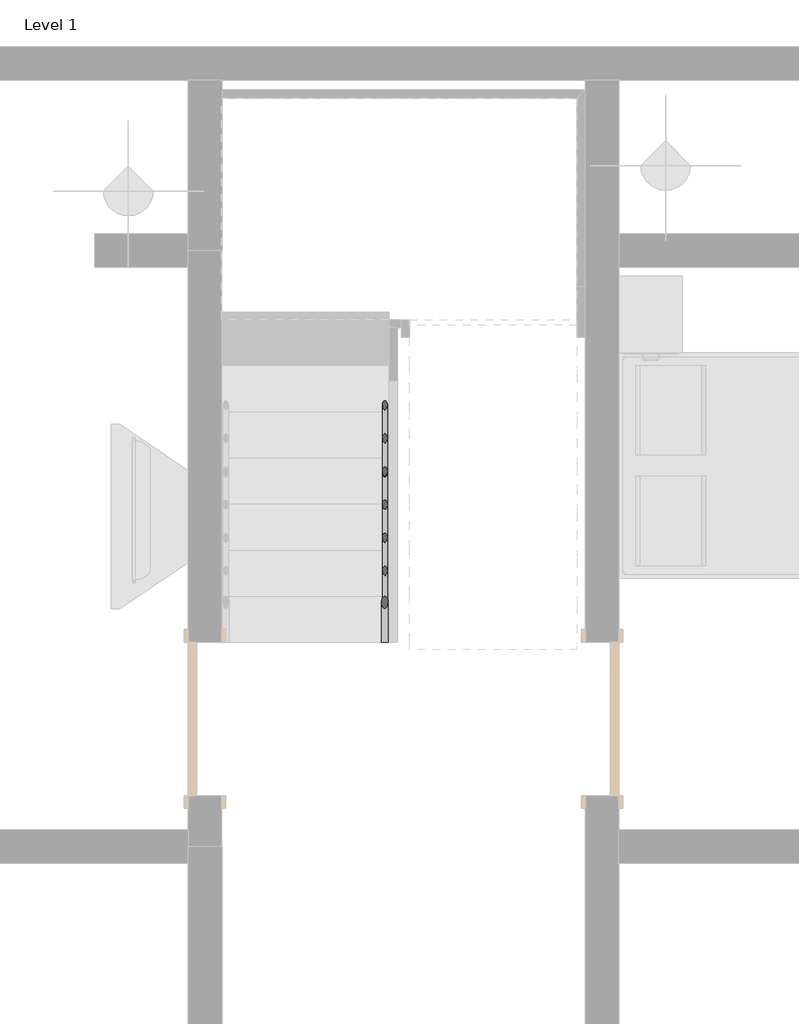
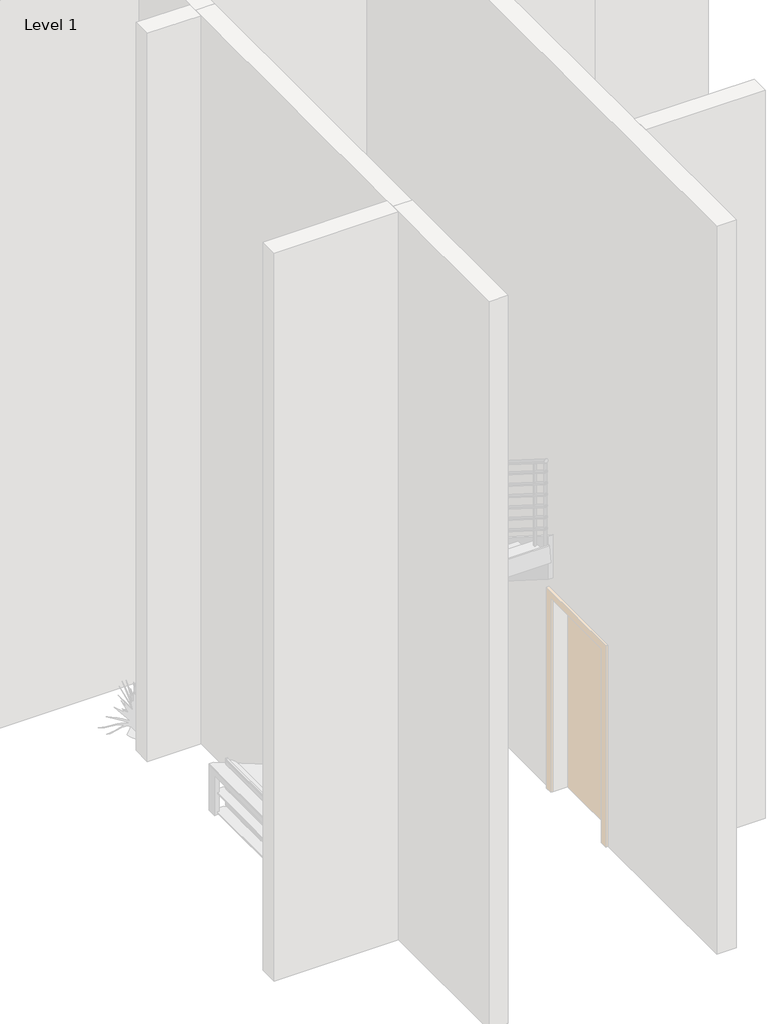
# One storey, part 2 of 4: 1 railing.
"""IFC4 building model written with IfcOpenShell, lengths in millimetres."""

from ifc_helpers import new_model, si_unit, point, frame, frame_2d, origin, place, context, project, spatial, circle_curve, ellipse_curve, trimmed, segment, composite_curve, outline, extrude, element, save
from ifc_brep_helpers import plane_surface, cylinder_surface, advanced_brep

model = new_model("IFC4")

# Units and contexts
model_context = context("Model", 3, world=origin())
ifc_project = project(units=[si_unit("LENGTHUNIT", "METRE", prefix="MILLI")], contexts=[model_context])

# Site, building, storey
site = spatial("IfcSite", under=ifc_project)
building = spatial("IfcBuilding", under=site)
storey = spatial("IfcBuildingStorey", under=building, Name="Level 1", Elevation=0.0)

# Railing
placement = place(None, origin())
element("IfcRailing", 1, ObjectType="900mm Pipe", at=placement, inside=storey, context=model_context, shape_type="SolidModel", body=[
    advanced_brep(
    [(-3568.2939506, 8898.7482221, 1050.2491997), (-3608.2939506, 8898.7482221, 1050.2491997), (-3568.2939506, 10842.9347103, 2279.7742515), (-3608.2939506, 10876.7415595, 2301.1540771)],
    [
        (0, 1, ellipse_curve(frame((-3588.2939506, 8898.7482221, 1050.2491997), z_axis=(0.0, -1.0, 0.0), x_axis=(0.0, 0.0, -1.0)), 23.6638438, 20.0)),
        (1, 0, ellipse_curve(frame((-3588.2939506, 8898.7482221, 1050.2491997), z_axis=(0.0, -1.0, 0.0), x_axis=(0.0, 0.0, -1.0)), 23.6638438, 20.0)),
        (2, 3, ellipse_curve(frame((-3588.2939506, 10859.8381349, 2290.4641643), z_axis=(0.7071067811865479, 0.5976263089853412, 0.37794549184843723), x_axis=(0.7071067811865474, -0.5976263089853417, -0.37794549184843734)), 28.2842712, 20.0)),
        (3, 2, ellipse_curve(frame((-3588.2939506, 10859.8381349, 2290.4641643), z_axis=(0.7071067811865479, 0.5976263089853412, 0.37794549184843723), x_axis=(0.7071067811865474, -0.5976263089853417, -0.37794549184843734)), 28.2842712, 20.0)),
        (0, 2),
        (3, 1),
    ],
    [
        plane_surface(frame((-3588.2939506, 8898.7482221, 1073.9130435), z_axis=(0.0, -1.0, 0.0), x_axis=(0.0, 0.0, 1.0))),
        plane_surface(frame((-3588.2939506, 10849.1482221, 2307.3675889), z_axis=(0.7071067811865479, 0.5976263089853412, 0.37794549184843723), x_axis=(0.7071067811865472, -0.5976263089853417, -0.37794549184843756))),
        cylinder_surface(frame((-3588.2939506, 8909.4381349, 1057.0096189), z_axis=(0.0, -0.8451712313980438, -0.5344956404098301), x_axis=(-1.0, 0.0, 0.0)), 20.0),
    ],
    [
        (0, [[1, 2]]),
        (1, [[3, 4]]),
        (2, [[-1, 5, -4, 6]]),
        (2, [[-2, -6, -3, -5]]),
    ],
),
    advanced_brep(
    [(-3560.7006131, 10829.1482221, 2271.3043478), (-3594.5074624, 10869.1482221, 2271.3043478), (-3414.8939506, 10829.1482221, 2271.3043478), (-3414.8939506, 10869.1482221, 2271.3043478)],
    [
        (0, 1, ellipse_curve(frame((-3577.6040377, 10849.1482221, 2271.3043478), z_axis=(-0.7071067811865479, -0.5976263089853412, -0.37794549184843723), x_axis=(-0.707106781186547, 0.5976263089853417, 0.37794549184843756)), 28.2842712, 20.0)),
        (1, 0, ellipse_curve(frame((-3577.6040377, 10849.1482221, 2271.3043478), z_axis=(-0.7071067811865479, -0.5976263089853412, -0.37794549184843723), x_axis=(-0.707106781186547, 0.5976263089853417, 0.37794549184843756)), 28.2842712, 20.0)),
        (2, 3, ellipse_curve(frame((-3414.8939506, 10849.1482221, 2271.3043478), z_axis=(0.7071067811865476, 0.0, 0.7071067811865476), x_axis=(-0.7071067811865474, 0.0, 0.7071067811865476)), 28.2842712, 20.0)),
        (3, 2, ellipse_curve(frame((-3414.8939506, 10849.1482221, 2271.3043478), z_axis=(0.7071067811865476, 0.0, 0.7071067811865476), x_axis=(-0.7071067811865474, 0.0, 0.7071067811865476)), 28.2842712, 20.0)),
        (0, 2),
        (3, 1),
    ],
    [
        plane_surface(frame((-3588.2939506, 10849.1482221, 2291.3043478), z_axis=(-0.7071067811865479, -0.5976263089853412, -0.37794549184843723), x_axis=(0.7071067811865472, -0.5976263089853417, -0.37794549184843756))),
        plane_surface(frame((-3434.8939506, 10849.1482221, 2291.3043478), z_axis=(0.7071067811865476, 0.0, 0.7071067811865476), x_axis=(0.7071067811865476, 0.0, -0.7071067811865476))),
        cylinder_surface(frame((-3588.2939506, 10849.1482221, 2271.3043478), z_axis=(-1.0, 0.0, 0.0), x_axis=(0.0, 1.0, 0.0)), 20.0),
    ],
    [
        (0, [[1, 2]]),
        (1, [[3, 4]]),
        (2, [[-1, 5, -4, 6]]),
        (2, [[-2, -6, -3, -5]]),
    ],
),
    advanced_brep(
    [(-3414.8939506, 10829.1482221, 2271.3043478), (-3414.8939506, 10869.1482221, 2271.3043478), (-3414.8939506, 10829.1482221, 2414.474684), (-3414.8939506, 10869.1482221, 2436.5059289)],
    [
        (0, 1, ellipse_curve(frame((-3414.8939506, 10849.1482221, 2271.3043478), z_axis=(-0.7071067811865476, 0.0, -0.7071067811865476), x_axis=(0.7071067811865476, 0.0, -0.7071067811865474)), 28.2842712, 20.0)),
        (1, 0, ellipse_curve(frame((-3414.8939506, 10849.1482221, 2271.3043478), z_axis=(-0.7071067811865476, 0.0, -0.7071067811865476), x_axis=(0.7071067811865476, 0.0, -0.7071067811865474)), 28.2842712, 20.0)),
        (2, 3, ellipse_curve(frame((-3414.8939506, 10849.1482221, 2425.4903064), z_axis=(0.0, -0.482443965445817, 0.8759268349610687), x_axis=(0.0, -0.8759268349610687, -0.48244396544581697)), 22.8329573, 20.0)),
        (3, 2, ellipse_curve(frame((-3414.8939506, 10849.1482221, 2425.4903064), z_axis=(0.0, -0.482443965445817, 0.8759268349610687), x_axis=(0.0, -0.8759268349610687, -0.48244396544581697)), 22.8329573, 20.0)),
        (0, 2),
        (3, 1),
    ],
    [
        plane_surface(frame((-3414.8939506, 10849.1482221, 2271.3043478), z_axis=(-0.7071067811865476, 0.0, -0.7071067811865476), x_axis=(0.7071067811865476, 0.0, -0.7071067811865476))),
        plane_surface(frame((-3414.8939506, 10849.1482221, 2425.4903064), z_axis=(0.0, -0.482443965445817, 0.8759268349610687), x_axis=(1.0, 0.0, 0.0))),
        cylinder_surface(frame((-3414.8939506, 10849.1482221, 2271.3043478), z_axis=(0.0, 0.0, -1.0), x_axis=(0.0, 1.0, 0.0)), 20.0),
    ],
    [
        (0, [[1, 2]]),
        (1, [[3, 4]]),
        (2, [[-1, 5, -4, 6]]),
        (2, [[-2, -6, -3, -5]]),
    ],
),
    advanced_brep(
    [(-3434.8939506, 10849.1482221, 2425.4903064), (-3394.8939506, 10849.1482221, 2425.4903064), (-3434.8939506, 8898.7482221, 3658.9448519), (-3394.8939506, 8898.7482221, 3658.9448519)],
    [
        (0, 1, ellipse_curve(frame((-3414.8939506, 10849.1482221, 2425.4903064), z_axis=(0.0, 0.482443965445817, -0.8759268349610687), x_axis=(0.0, 0.8759268349610686, 0.48244396544581697)), 22.8329573, 20.0)),
        (1, 0, ellipse_curve(frame((-3414.8939506, 10849.1482221, 2425.4903064), z_axis=(0.0, 0.482443965445817, -0.8759268349610687), x_axis=(0.0, 0.8759268349610686, 0.48244396544581697)), 22.8329573, 20.0)),
        (2, 3, ellipse_curve(frame((-3414.8939506, 8898.7482221, 3658.9448519), z_axis=(0.0, -1.0, 0.0), x_axis=(0.0, 0.0, -1.0)), 23.6638438, 20.0)),
        (3, 2, ellipse_curve(frame((-3414.8939506, 8898.7482221, 3658.9448519), z_axis=(0.0, -1.0, 0.0), x_axis=(0.0, 0.0, -1.0)), 23.6638438, 20.0)),
        (0, 2),
        (3, 1),
    ],
    [
        plane_surface(frame((-3414.8939506, 10869.1482221, 2436.5059289), z_axis=(0.0, 0.482443965445817, -0.8759268349610687), x_axis=(1.0, 0.0, 0.0))),
        plane_surface(frame((-3414.8939506, 8898.7482221, 3682.6086957), z_axis=(0.0, -1.0, 0.0), x_axis=(0.0, 0.0, -1.0))),
        cylinder_surface(frame((-3414.8939506, 10858.4583093, 2419.6025042), z_axis=(0.0, 0.8451712313980434, -0.5344956404098308), x_axis=(1.0, 0.0, 0.0)), 20.0),
    ],
    [
        (0, [[1, 2]]),
        (1, [[3, 4]]),
        (2, [[-1, 5, -4, 6]]),
        (2, [[-2, -6, -3, -5]]),
    ],
),
    advanced_brep(
    [(-3603.2939506, 8898.7482221, 931.1651606), (-3573.2939506, 8898.7482221, 931.1651606), (-3603.2939506, 10828.0933118, 2151.3043478), (-3573.2939506, 10828.0933118, 2151.3043478), (-3603.2939506, 10864.1482221, 2151.3043478), (-3573.2939506, 10834.1482221, 2151.3043478), (-3429.8939506, 10864.1482221, 2151.3043478), (-3429.8939506, 10834.1482221, 2151.3043478)],
    [
        (0, 1, ellipse_curve(frame((-3588.2939506, 8898.7482221, 931.1651606), z_axis=(0.0, -1.0, 0.0), x_axis=(0.0, 0.0, -1.0)), 17.7478828, 15.0)),
        (1, 0, ellipse_curve(frame((-3588.2939506, 8898.7482221, 931.1651606), z_axis=(0.0, -1.0, 0.0), x_axis=(0.0, 0.0, -1.0)), 17.7478828, 15.0)),
        (0, 2),
        (2, 3, ellipse_curve(frame((-3588.2939506, 10828.0933118, 2151.3043478), z_axis=(0.0, -0.9605132043335073, -0.2782344053149755), x_axis=(0.0, 0.27823440531497556, -0.9605132043335073)), 15.6166515, 15.0)),
        (3, 1),
        (3, 2, ellipse_curve(frame((-3588.2939506, 10828.0933118, 2151.3043478), z_axis=(0.0, -0.9605132043335073, -0.2782344053149755), x_axis=(0.0, 0.27823440531497556, -0.9605132043335073)), 15.6166515, 15.0)),
        (2, 4),
        (4, 5, ellipse_curve(frame((-3588.2939506, 10849.1482221, 2151.3043478), z_axis=(-0.7071067811865479, -0.707106781186547, 0.0), x_axis=(0.707106781186547, -0.707106781186548, 0.0)), 21.2132034, 15.0)),
        (5, 3),
        (5, 4, ellipse_curve(frame((-3588.2939506, 10849.1482221, 2151.3043478), z_axis=(-0.7071067811865479, -0.707106781186547, 0.0), x_axis=(0.707106781186547, -0.707106781186548, 0.0)), 21.2132034, 15.0)),
        (6, 7, circle_curve(frame((-3429.8939506, 10849.1482221, 2151.3043478), z_axis=(1.0, 0.0, 0.0), x_axis=(0.0, -1.0, 0.0)), 15.0)),
        (7, 6, circle_curve(frame((-3429.8939506, 10849.1482221, 2151.3043478), z_axis=(1.0, 0.0, 0.0), x_axis=(0.0, -1.0, 0.0)), 15.0)),
        (4, 6),
        (7, 5),
    ],
    [
        plane_surface(frame((-3588.2939506, 8898.7482221, 948.9130435), z_axis=(0.0, -1.0, 0.0), x_axis=(0.0, 0.0, 1.0))),
        cylinder_surface(frame((-3588.2939506, 8906.7656567, 936.235475), z_axis=(0.0, -0.8451712313980438, -0.5344956404098301), x_axis=(1.0, 0.0, 0.0)), 15.0),
        cylinder_surface(frame((-3588.2939506, 10823.7482221, 2151.3043478), z_axis=(0.0, -1.0, 0.0), x_axis=(1.0, 0.0, 0.0)), 15.0),
        plane_surface(frame((-3429.8939506, 10849.1482221, 2166.3043478), z_axis=(1.0, 0.0, 0.0), x_axis=(0.0, 1.0, 0.0))),
        cylinder_surface(frame((-3588.2939506, 10849.1482221, 2151.3043478), z_axis=(-1.0, 0.0, 0.0), x_axis=(0.0, -1.0, 0.0)), 15.0),
    ],
    [
        (0, [[1, 2]]),
        (1, [[-1, 3, 4, 5]]),
        (1, [[-2, -5, 6, -3]]),
        (2, [[-4, 7, 8, 9]]),
        (2, [[-6, -9, 10, -7]]),
        (3, [[11, 12]]),
        (4, [[-8, 13, -12, 14]]),
        (4, [[-10, -14, -11, -13]]),
    ],
),
    advanced_brep(
    [(-3399.8939506, 10864.1482221, 2296.9201013), (-3429.8939506, 10864.1482221, 2296.9201013), (-3399.8939506, 8898.7482221, 3539.8608128), (-3429.8939506, 8898.7482221, 3539.8608128)],
    [
        (0, 1, ellipse_curve(frame((-3414.8939506, 10864.1482221, 2296.9201013), z_axis=(0.0, 1.0, 0.0), x_axis=(0.0, 0.0, -1.0)), 17.7478828, 15.0)),
        (1, 0, ellipse_curve(frame((-3414.8939506, 10864.1482221, 2296.9201013), z_axis=(0.0, 1.0, 0.0), x_axis=(0.0, 0.0, -1.0)), 17.7478828, 15.0)),
        (2, 3, ellipse_curve(frame((-3414.8939506, 8898.7482221, 3539.8608128), z_axis=(0.0, -1.0, 0.0), x_axis=(0.0, 0.0, -1.0)), 17.7478828, 15.0)),
        (3, 2, ellipse_curve(frame((-3414.8939506, 8898.7482221, 3539.8608128), z_axis=(0.0, -1.0, 0.0), x_axis=(0.0, 0.0, -1.0)), 17.7478828, 15.0)),
        (0, 2),
        (3, 1),
    ],
    [
        plane_surface(frame((-3414.8939506, 10864.1482221, 2314.6679842), z_axis=(0.0, 1.0, 0.0), x_axis=(0.0, 0.0, -1.0))),
        plane_surface(frame((-3414.8939506, 8898.7482221, 3557.6086957), z_axis=(0.0, -1.0, 0.0), x_axis=(0.0, 0.0, -1.0))),
        cylinder_surface(frame((-3414.8939506, 10856.1307875, 2301.9904157), z_axis=(0.0, 0.8451712313980434, -0.5344956404098308), x_axis=(-1.0, 0.0, 0.0)), 15.0),
    ],
    [
        (0, [[1, 2]]),
        (1, [[3, 4]]),
        (2, [[-1, 5, -4, 6]]),
        (2, [[-2, -6, -3, -5]]),
    ],
),
    advanced_brep(
    [(-3603.2939506, 8898.7482221, 806.1651606), (-3573.2939506, 8898.7482221, 806.1651606), (-3603.2939506, 10828.0933118, 2026.3043478), (-3573.2939506, 10828.0933118, 2026.3043478), (-3603.2939506, 10864.1482221, 2026.3043478), (-3573.2939506, 10834.1482221, 2026.3043478), (-3429.8939506, 10864.1482221, 2026.3043478), (-3429.8939506, 10834.1482221, 2026.3043478)],
    [
        (0, 1, ellipse_curve(frame((-3588.2939506, 8898.7482221, 806.1651606), z_axis=(0.0, -1.0, 0.0), x_axis=(0.0, 0.0, -1.0)), 17.7478828, 15.0)),
        (1, 0, ellipse_curve(frame((-3588.2939506, 8898.7482221, 806.1651606), z_axis=(0.0, -1.0, 0.0), x_axis=(0.0, 0.0, -1.0)), 17.7478828, 15.0)),
        (0, 2),
        (2, 3, ellipse_curve(frame((-3588.2939506, 10828.0933118, 2026.3043478), z_axis=(0.0, -0.9605132043335073, -0.2782344053149755), x_axis=(0.0, 0.27823440531497556, -0.9605132043335073)), 15.6166515, 15.0)),
        (3, 1),
        (3, 2, ellipse_curve(frame((-3588.2939506, 10828.0933118, 2026.3043478), z_axis=(0.0, -0.9605132043335073, -0.2782344053149755), x_axis=(0.0, 0.27823440531497556, -0.9605132043335073)), 15.6166515, 15.0)),
        (2, 4),
        (4, 5, ellipse_curve(frame((-3588.2939506, 10849.1482221, 2026.3043478), z_axis=(-0.7071067811865479, -0.707106781186547, 0.0), x_axis=(0.707106781186547, -0.707106781186548, 0.0)), 21.2132034, 15.0)),
        (5, 3),
        (5, 4, ellipse_curve(frame((-3588.2939506, 10849.1482221, 2026.3043478), z_axis=(-0.7071067811865479, -0.707106781186547, 0.0), x_axis=(0.707106781186547, -0.707106781186548, 0.0)), 21.2132034, 15.0)),
        (6, 7, circle_curve(frame((-3429.8939506, 10849.1482221, 2026.3043478), z_axis=(1.0, 0.0, 0.0), x_axis=(0.0, -1.0, 0.0)), 15.0)),
        (7, 6, circle_curve(frame((-3429.8939506, 10849.1482221, 2026.3043478), z_axis=(1.0, 0.0, 0.0), x_axis=(0.0, -1.0, 0.0)), 15.0)),
        (4, 6),
        (7, 5),
    ],
    [
        plane_surface(frame((-3588.2939506, 8898.7482221, 823.9130435), z_axis=(0.0, -1.0, 0.0), x_axis=(0.0, 0.0, 1.0))),
        cylinder_surface(frame((-3588.2939506, 8906.7656567, 811.235475), z_axis=(0.0, -0.8451712313980438, -0.5344956404098301), x_axis=(1.0, 0.0, 0.0)), 15.0),
        cylinder_surface(frame((-3588.2939506, 10823.7482221, 2026.3043478), z_axis=(0.0, -1.0, 0.0), x_axis=(1.0, 0.0, 0.0)), 15.0),
        plane_surface(frame((-3429.8939506, 10849.1482221, 2041.3043478), z_axis=(1.0, 0.0, 0.0), x_axis=(0.0, 1.0, 0.0))),
        cylinder_surface(frame((-3588.2939506, 10849.1482221, 2026.3043478), z_axis=(-1.0, 0.0, 0.0), x_axis=(0.0, -1.0, 0.0)), 15.0),
    ],
    [
        (0, [[1, 2]]),
        (1, [[-1, 3, 4, 5]]),
        (1, [[-2, -5, 6, -3]]),
        (2, [[-4, 7, 8, 9]]),
        (2, [[-6, -9, 10, -7]]),
        (3, [[11, 12]]),
        (4, [[-8, 13, -12, 14]]),
        (4, [[-10, -14, -11, -13]]),
    ],
),
    advanced_brep(
    [(-3399.8939506, 10864.1482221, 2171.9201013), (-3429.8939506, 10864.1482221, 2171.9201013), (-3399.8939506, 8898.7482221, 3414.8608128), (-3429.8939506, 8898.7482221, 3414.8608128)],
    [
        (0, 1, ellipse_curve(frame((-3414.8939506, 10864.1482221, 2171.9201013), z_axis=(0.0, 1.0, 0.0), x_axis=(0.0, 0.0, -1.0)), 17.7478828, 15.0)),
        (1, 0, ellipse_curve(frame((-3414.8939506, 10864.1482221, 2171.9201013), z_axis=(0.0, 1.0, 0.0), x_axis=(0.0, 0.0, -1.0)), 17.7478828, 15.0)),
        (2, 3, ellipse_curve(frame((-3414.8939506, 8898.7482221, 3414.8608128), z_axis=(0.0, -1.0, 0.0), x_axis=(0.0, 0.0, -1.0)), 17.7478828, 15.0)),
        (3, 2, ellipse_curve(frame((-3414.8939506, 8898.7482221, 3414.8608128), z_axis=(0.0, -1.0, 0.0), x_axis=(0.0, 0.0, -1.0)), 17.7478828, 15.0)),
        (0, 2),
        (3, 1),
    ],
    [
        plane_surface(frame((-3414.8939506, 10864.1482221, 2189.6679842), z_axis=(0.0, 1.0, 0.0), x_axis=(0.0, 0.0, -1.0))),
        plane_surface(frame((-3414.8939506, 8898.7482221, 3432.6086957), z_axis=(0.0, -1.0, 0.0), x_axis=(0.0, 0.0, -1.0))),
        cylinder_surface(frame((-3414.8939506, 10856.1307875, 2176.9904157), z_axis=(0.0, 0.8451712313980434, -0.5344956404098307), x_axis=(-1.0, 0.0, 0.0)), 15.0),
    ],
    [
        (0, [[1, 2]]),
        (1, [[3, 4]]),
        (2, [[-1, 5, -4, 6]]),
        (2, [[-2, -6, -3, -5]]),
    ],
),
    advanced_brep(
    [(-3603.2939506, 8898.7482221, 681.1651606), (-3573.2939506, 8898.7482221, 681.1651606), (-3603.2939506, 10828.0933118, 1901.3043478), (-3573.2939506, 10828.0933118, 1901.3043478), (-3603.2939506, 10864.1482221, 1901.3043478), (-3573.2939506, 10834.1482221, 1901.3043478), (-3429.8939506, 10864.1482221, 1901.3043478), (-3429.8939506, 10834.1482221, 1901.3043478)],
    [
        (0, 1, ellipse_curve(frame((-3588.2939506, 8898.7482221, 681.1651606), z_axis=(0.0, -1.0, 0.0), x_axis=(0.0, 0.0, -1.0)), 17.7478828, 15.0)),
        (1, 0, ellipse_curve(frame((-3588.2939506, 8898.7482221, 681.1651606), z_axis=(0.0, -1.0, 0.0), x_axis=(0.0, 0.0, -1.0)), 17.7478828, 15.0)),
        (0, 2),
        (2, 3, ellipse_curve(frame((-3588.2939506, 10828.0933118, 1901.3043478), z_axis=(0.0, -0.9605132043335073, -0.2782344053149755), x_axis=(0.0, 0.27823440531497556, -0.9605132043335073)), 15.6166515, 15.0)),
        (3, 1),
        (3, 2, ellipse_curve(frame((-3588.2939506, 10828.0933118, 1901.3043478), z_axis=(0.0, -0.9605132043335073, -0.2782344053149755), x_axis=(0.0, 0.27823440531497556, -0.9605132043335073)), 15.6166515, 15.0)),
        (2, 4),
        (4, 5, ellipse_curve(frame((-3588.2939506, 10849.1482221, 1901.3043478), z_axis=(-0.7071067811865479, -0.707106781186547, 0.0), x_axis=(0.707106781186547, -0.707106781186548, 0.0)), 21.2132034, 15.0)),
        (5, 3),
        (5, 4, ellipse_curve(frame((-3588.2939506, 10849.1482221, 1901.3043478), z_axis=(-0.7071067811865479, -0.707106781186547, 0.0), x_axis=(0.707106781186547, -0.707106781186548, 0.0)), 21.2132034, 15.0)),
        (6, 7, circle_curve(frame((-3429.8939506, 10849.1482221, 1901.3043478), z_axis=(1.0, 0.0, 0.0), x_axis=(0.0, -1.0, 0.0)), 15.0)),
        (7, 6, circle_curve(frame((-3429.8939506, 10849.1482221, 1901.3043478), z_axis=(1.0, 0.0, 0.0), x_axis=(0.0, -1.0, 0.0)), 15.0)),
        (4, 6),
        (7, 5),
    ],
    [
        plane_surface(frame((-3588.2939506, 8898.7482221, 698.9130435), z_axis=(0.0, -1.0, 0.0), x_axis=(0.0, 0.0, 1.0))),
        cylinder_surface(frame((-3588.2939506, 8906.7656567, 686.235475), z_axis=(0.0, -0.8451712313980438, -0.5344956404098301), x_axis=(1.0, 0.0, 0.0)), 15.0),
        cylinder_surface(frame((-3588.2939506, 10823.7482221, 1901.3043478), z_axis=(0.0, -1.0, 0.0), x_axis=(1.0, 0.0, 0.0)), 15.0),
        plane_surface(frame((-3429.8939506, 10849.1482221, 1916.3043478), z_axis=(1.0, 0.0, 0.0), x_axis=(0.0, 1.0, 0.0))),
        cylinder_surface(frame((-3588.2939506, 10849.1482221, 1901.3043478), z_axis=(-1.0, 0.0, 0.0), x_axis=(0.0, -1.0, 0.0)), 15.0),
    ],
    [
        (0, [[1, 2]]),
        (1, [[-1, 3, 4, 5]]),
        (1, [[-2, -5, 6, -3]]),
        (2, [[-4, 7, 8, 9]]),
        (2, [[-6, -9, 10, -7]]),
        (3, [[11, 12]]),
        (4, [[-8, 13, -12, 14]]),
        (4, [[-10, -14, -11, -13]]),
    ],
),
    advanced_brep(
    [(-3399.8939506, 10864.1482221, 2046.9201013), (-3429.8939506, 10864.1482221, 2046.9201013), (-3399.8939506, 8898.7482221, 3289.8608128), (-3429.8939506, 8898.7482221, 3289.8608128)],
    [
        (0, 1, ellipse_curve(frame((-3414.8939506, 10864.1482221, 2046.9201013), z_axis=(0.0, 1.0, 0.0), x_axis=(0.0, 0.0, -1.0)), 17.7478828, 15.0)),
        (1, 0, ellipse_curve(frame((-3414.8939506, 10864.1482221, 2046.9201013), z_axis=(0.0, 1.0, 0.0), x_axis=(0.0, 0.0, -1.0)), 17.7478828, 15.0)),
        (2, 3, ellipse_curve(frame((-3414.8939506, 8898.7482221, 3289.8608128), z_axis=(0.0, -1.0, 0.0), x_axis=(0.0, 0.0, -1.0)), 17.7478828, 15.0)),
        (3, 2, ellipse_curve(frame((-3414.8939506, 8898.7482221, 3289.8608128), z_axis=(0.0, -1.0, 0.0), x_axis=(0.0, 0.0, -1.0)), 17.7478828, 15.0)),
        (0, 2),
        (3, 1),
    ],
    [
        plane_surface(frame((-3414.8939506, 10864.1482221, 2064.6679842), z_axis=(0.0, 1.0, 0.0), x_axis=(0.0, 0.0, -1.0))),
        plane_surface(frame((-3414.8939506, 8898.7482221, 3307.6086957), z_axis=(0.0, -1.0, 0.0), x_axis=(0.0, 0.0, -1.0))),
        cylinder_surface(frame((-3414.8939506, 10856.1307875, 2051.9904157), z_axis=(0.0, 0.8451712313980435, -0.5344956404098306), x_axis=(-1.0, 0.0, 0.0)), 15.0),
    ],
    [
        (0, [[1, 2]]),
        (1, [[3, 4]]),
        (2, [[-1, 5, -4, 6]]),
        (2, [[-2, -6, -3, -5]]),
    ],
),
    advanced_brep(
    [(-3603.2939506, 8898.7482221, 556.1651606), (-3573.2939506, 8898.7482221, 556.1651606), (-3603.2939506, 10828.0933118, 1776.3043478), (-3573.2939506, 10828.0933118, 1776.3043478), (-3603.2939506, 10864.1482221, 1776.3043478), (-3573.2939506, 10834.1482221, 1776.3043478), (-3429.8939506, 10864.1482221, 1776.3043478), (-3429.8939506, 10834.1482221, 1776.3043478)],
    [
        (0, 1, ellipse_curve(frame((-3588.2939506, 8898.7482221, 556.1651606), z_axis=(0.0, -1.0, 0.0), x_axis=(0.0, 0.0, -1.0)), 17.7478828, 15.0)),
        (1, 0, ellipse_curve(frame((-3588.2939506, 8898.7482221, 556.1651606), z_axis=(0.0, -1.0, 0.0), x_axis=(0.0, 0.0, -1.0)), 17.7478828, 15.0)),
        (0, 2),
        (2, 3, ellipse_curve(frame((-3588.2939506, 10828.0933118, 1776.3043478), z_axis=(0.0, -0.9605132043335073, -0.2782344053149755), x_axis=(0.0, 0.27823440531497556, -0.9605132043335073)), 15.6166515, 15.0)),
        (3, 1),
        (3, 2, ellipse_curve(frame((-3588.2939506, 10828.0933118, 1776.3043478), z_axis=(0.0, -0.9605132043335073, -0.2782344053149755), x_axis=(0.0, 0.27823440531497556, -0.9605132043335073)), 15.6166515, 15.0)),
        (2, 4),
        (4, 5, ellipse_curve(frame((-3588.2939506, 10849.1482221, 1776.3043478), z_axis=(-0.7071067811865479, -0.707106781186547, 0.0), x_axis=(0.707106781186547, -0.707106781186548, 0.0)), 21.2132034, 15.0)),
        (5, 3),
        (5, 4, ellipse_curve(frame((-3588.2939506, 10849.1482221, 1776.3043478), z_axis=(-0.7071067811865479, -0.707106781186547, 0.0), x_axis=(0.707106781186547, -0.707106781186548, 0.0)), 21.2132034, 15.0)),
        (6, 7, circle_curve(frame((-3429.8939506, 10849.1482221, 1776.3043478), z_axis=(1.0, 0.0, 0.0), x_axis=(0.0, -1.0, 0.0)), 15.0)),
        (7, 6, circle_curve(frame((-3429.8939506, 10849.1482221, 1776.3043478), z_axis=(1.0, 0.0, 0.0), x_axis=(0.0, -1.0, 0.0)), 15.0)),
        (4, 6),
        (7, 5),
    ],
    [
        plane_surface(frame((-3588.2939506, 8898.7482221, 573.9130435), z_axis=(0.0, -1.0, 0.0), x_axis=(0.0, 0.0, 1.0))),
        cylinder_surface(frame((-3588.2939506, 8906.7656567, 561.235475), z_axis=(0.0, -0.8451712313980438, -0.5344956404098301), x_axis=(1.0, 0.0, 0.0)), 15.0),
        cylinder_surface(frame((-3588.2939506, 10823.7482221, 1776.3043478), z_axis=(0.0, -1.0, 0.0), x_axis=(1.0, 0.0, 0.0)), 15.0),
        plane_surface(frame((-3429.8939506, 10849.1482221, 1791.3043478), z_axis=(1.0, 0.0, 0.0), x_axis=(0.0, 1.0, 0.0))),
        cylinder_surface(frame((-3588.2939506, 10849.1482221, 1776.3043478), z_axis=(-1.0, 0.0, 0.0), x_axis=(0.0, -1.0, 0.0)), 15.0),
    ],
    [
        (0, [[1, 2]]),
        (1, [[-1, 3, 4, 5]]),
        (1, [[-2, -5, 6, -3]]),
        (2, [[-4, 7, 8, 9]]),
        (2, [[-6, -9, 10, -7]]),
        (3, [[11, 12]]),
        (4, [[-8, 13, -12, 14]]),
        (4, [[-10, -14, -11, -13]]),
    ],
),
    advanced_brep(
    [(-3399.8939506, 10864.1482221, 1921.9201013), (-3429.8939506, 10864.1482221, 1921.9201013), (-3399.8939506, 8898.7482221, 3164.8608128), (-3429.8939506, 8898.7482221, 3164.8608128)],
    [
        (0, 1, ellipse_curve(frame((-3414.8939506, 10864.1482221, 1921.9201013), z_axis=(0.0, 1.0, 0.0), x_axis=(0.0, 0.0, -1.0)), 17.7478828, 15.0)),
        (1, 0, ellipse_curve(frame((-3414.8939506, 10864.1482221, 1921.9201013), z_axis=(0.0, 1.0, 0.0), x_axis=(0.0, 0.0, -1.0)), 17.7478828, 15.0)),
        (2, 3, ellipse_curve(frame((-3414.8939506, 8898.7482221, 3164.8608128), z_axis=(0.0, -1.0, 0.0), x_axis=(0.0, 0.0, -1.0)), 17.7478828, 15.0)),
        (3, 2, ellipse_curve(frame((-3414.8939506, 8898.7482221, 3164.8608128), z_axis=(0.0, -1.0, 0.0), x_axis=(0.0, 0.0, -1.0)), 17.7478828, 15.0)),
        (0, 2),
        (3, 1),
    ],
    [
        plane_surface(frame((-3414.8939506, 10864.1482221, 1939.6679842), z_axis=(0.0, 1.0, 0.0), x_axis=(0.0, 0.0, -1.0))),
        plane_surface(frame((-3414.8939506, 8898.7482221, 3182.6086957), z_axis=(0.0, -1.0, 0.0), x_axis=(0.0, 0.0, -1.0))),
        cylinder_surface(frame((-3414.8939506, 10856.1307875, 1926.9904157), z_axis=(0.0, 0.8451712313980434, -0.5344956404098307), x_axis=(-1.0, 0.0, 0.0)), 15.0),
    ],
    [
        (0, [[1, 2]]),
        (1, [[3, 4]]),
        (2, [[-1, 5, -4, 6]]),
        (2, [[-2, -6, -3, -5]]),
    ],
),
    advanced_brep(
    [(-3603.2939506, 8898.7482221, 431.1651606), (-3573.2939506, 8898.7482221, 431.1651606), (-3603.2939506, 10828.0933118, 1651.3043478), (-3573.2939506, 10828.0933118, 1651.3043478), (-3603.2939506, 10864.1482221, 1651.3043478), (-3573.2939506, 10834.1482221, 1651.3043478), (-3429.8939506, 10864.1482221, 1651.3043478), (-3429.8939506, 10834.1482221, 1651.3043478)],
    [
        (0, 1, ellipse_curve(frame((-3588.2939506, 8898.7482221, 431.1651606), z_axis=(0.0, -1.0, 0.0), x_axis=(0.0, 0.0, -1.0)), 17.7478828, 15.0)),
        (1, 0, ellipse_curve(frame((-3588.2939506, 8898.7482221, 431.1651606), z_axis=(0.0, -1.0, 0.0), x_axis=(0.0, 0.0, -1.0)), 17.7478828, 15.0)),
        (0, 2),
        (2, 3, ellipse_curve(frame((-3588.2939506, 10828.0933118, 1651.3043478), z_axis=(0.0, -0.9605132043335073, -0.2782344053149755), x_axis=(0.0, 0.27823440531497556, -0.9605132043335073)), 15.6166515, 15.0)),
        (3, 1),
        (3, 2, ellipse_curve(frame((-3588.2939506, 10828.0933118, 1651.3043478), z_axis=(0.0, -0.9605132043335073, -0.2782344053149755), x_axis=(0.0, 0.27823440531497556, -0.9605132043335073)), 15.6166515, 15.0)),
        (2, 4),
        (4, 5, ellipse_curve(frame((-3588.2939506, 10849.1482221, 1651.3043478), z_axis=(-0.7071067811865479, -0.707106781186547, 0.0), x_axis=(0.707106781186547, -0.707106781186548, 0.0)), 21.2132034, 15.0)),
        (5, 3),
        (5, 4, ellipse_curve(frame((-3588.2939506, 10849.1482221, 1651.3043478), z_axis=(-0.7071067811865479, -0.707106781186547, 0.0), x_axis=(0.707106781186547, -0.707106781186548, 0.0)), 21.2132034, 15.0)),
        (6, 7, circle_curve(frame((-3429.8939506, 10849.1482221, 1651.3043478), z_axis=(1.0, 0.0, 0.0), x_axis=(0.0, -1.0, 0.0)), 15.0)),
        (7, 6, circle_curve(frame((-3429.8939506, 10849.1482221, 1651.3043478), z_axis=(1.0, 0.0, 0.0), x_axis=(0.0, -1.0, 0.0)), 15.0)),
        (4, 6),
        (7, 5),
    ],
    [
        plane_surface(frame((-3588.2939506, 8898.7482221, 448.9130435), z_axis=(0.0, -1.0, 0.0), x_axis=(0.0, 0.0, 1.0))),
        cylinder_surface(frame((-3588.2939506, 8906.7656567, 436.235475), z_axis=(0.0, -0.8451712313980438, -0.5344956404098301), x_axis=(1.0, 0.0, 0.0)), 15.0),
        cylinder_surface(frame((-3588.2939506, 10823.7482221, 1651.3043478), z_axis=(0.0, -1.0, 0.0), x_axis=(1.0, 0.0, 0.0)), 15.0),
        plane_surface(frame((-3429.8939506, 10849.1482221, 1666.3043478), z_axis=(1.0, 0.0, 0.0), x_axis=(0.0, 1.0, 0.0))),
        cylinder_surface(frame((-3588.2939506, 10849.1482221, 1651.3043478), z_axis=(-1.0, 0.0, 0.0), x_axis=(0.0, -1.0, 0.0)), 15.0),
    ],
    [
        (0, [[1, 2]]),
        (1, [[-1, 3, 4, 5]]),
        (1, [[-2, -5, 6, -3]]),
        (2, [[-4, 7, 8, 9]]),
        (2, [[-6, -9, 10, -7]]),
        (3, [[11, 12]]),
        (4, [[-8, 13, -12, 14]]),
        (4, [[-10, -14, -11, -13]]),
    ],
),
    advanced_brep(
    [(-3399.8939506, 10864.1482221, 1796.9201013), (-3429.8939506, 10864.1482221, 1796.9201013), (-3399.8939506, 8898.7482221, 3039.8608128), (-3429.8939506, 8898.7482221, 3039.8608128)],
    [
        (0, 1, ellipse_curve(frame((-3414.8939506, 10864.1482221, 1796.9201013), z_axis=(0.0, 1.0, 0.0), x_axis=(0.0, 0.0, -1.0)), 17.7478828, 15.0)),
        (1, 0, ellipse_curve(frame((-3414.8939506, 10864.1482221, 1796.9201013), z_axis=(0.0, 1.0, 0.0), x_axis=(0.0, 0.0, -1.0)), 17.7478828, 15.0)),
        (2, 3, ellipse_curve(frame((-3414.8939506, 8898.7482221, 3039.8608128), z_axis=(0.0, -1.0, 0.0), x_axis=(0.0, 0.0, -1.0)), 17.7478828, 15.0)),
        (3, 2, ellipse_curve(frame((-3414.8939506, 8898.7482221, 3039.8608128), z_axis=(0.0, -1.0, 0.0), x_axis=(0.0, 0.0, -1.0)), 17.7478828, 15.0)),
        (0, 2),
        (3, 1),
    ],
    [
        plane_surface(frame((-3414.8939506, 10864.1482221, 1814.6679842), z_axis=(0.0, 1.0, 0.0), x_axis=(0.0, 0.0, -1.0))),
        plane_surface(frame((-3414.8939506, 8898.7482221, 3057.6086957), z_axis=(0.0, -1.0, 0.0), x_axis=(0.0, 0.0, -1.0))),
        cylinder_surface(frame((-3414.8939506, 10856.1307875, 1801.9904157), z_axis=(0.0, 0.8451712313980434, -0.5344956404098308), x_axis=(-1.0, 0.0, 0.0)), 15.0),
    ],
    [
        (0, [[1, 2]]),
        (1, [[3, 4]]),
        (2, [[-1, 5, -4, 6]]),
        (2, [[-2, -6, -3, -5]]),
    ],
),
    advanced_brep(
    [(-3603.2939506, 8898.7482221, 306.1651606), (-3573.2939506, 8898.7482221, 306.1651606), (-3603.2939506, 10828.0933118, 1526.3043478), (-3573.2939506, 10828.0933118, 1526.3043478), (-3603.2939506, 10864.1482221, 1526.3043478), (-3573.2939506, 10834.1482221, 1526.3043478), (-3429.8939506, 10864.1482221, 1526.3043478), (-3429.8939506, 10834.1482221, 1526.3043478)],
    [
        (0, 1, ellipse_curve(frame((-3588.2939506, 8898.7482221, 306.1651606), z_axis=(0.0, -1.0, 0.0), x_axis=(0.0, 0.0, -1.0)), 17.7478828, 15.0)),
        (1, 0, ellipse_curve(frame((-3588.2939506, 8898.7482221, 306.1651606), z_axis=(0.0, -1.0, 0.0), x_axis=(0.0, 0.0, -1.0)), 17.7478828, 15.0)),
        (0, 2),
        (2, 3, ellipse_curve(frame((-3588.2939506, 10828.0933118, 1526.3043478), z_axis=(0.0, -0.9605132043335073, -0.2782344053149755), x_axis=(0.0, 0.27823440531497556, -0.9605132043335073)), 15.6166515, 15.0)),
        (3, 1),
        (3, 2, ellipse_curve(frame((-3588.2939506, 10828.0933118, 1526.3043478), z_axis=(0.0, -0.9605132043335073, -0.2782344053149755), x_axis=(0.0, 0.27823440531497556, -0.9605132043335073)), 15.6166515, 15.0)),
        (2, 4),
        (4, 5, ellipse_curve(frame((-3588.2939506, 10849.1482221, 1526.3043478), z_axis=(-0.7071067811865479, -0.707106781186547, 0.0), x_axis=(0.707106781186547, -0.707106781186548, 0.0)), 21.2132034, 15.0)),
        (5, 3),
        (5, 4, ellipse_curve(frame((-3588.2939506, 10849.1482221, 1526.3043478), z_axis=(-0.7071067811865479, -0.707106781186547, 0.0), x_axis=(0.707106781186547, -0.707106781186548, 0.0)), 21.2132034, 15.0)),
        (6, 7, circle_curve(frame((-3429.8939506, 10849.1482221, 1526.3043478), z_axis=(1.0, 0.0, 0.0), x_axis=(0.0, -1.0, 0.0)), 15.0)),
        (7, 6, circle_curve(frame((-3429.8939506, 10849.1482221, 1526.3043478), z_axis=(1.0, 0.0, 0.0), x_axis=(0.0, -1.0, 0.0)), 15.0)),
        (4, 6),
        (7, 5),
    ],
    [
        plane_surface(frame((-3588.2939506, 8898.7482221, 323.9130435), z_axis=(0.0, -1.0, 0.0), x_axis=(0.0, 0.0, 1.0))),
        cylinder_surface(frame((-3588.2939506, 8906.7656567, 311.235475), z_axis=(0.0, -0.8451712313980438, -0.5344956404098301), x_axis=(1.0, 0.0, 0.0)), 15.0),
        cylinder_surface(frame((-3588.2939506, 10823.7482221, 1526.3043478), z_axis=(0.0, -1.0, 0.0), x_axis=(1.0, 0.0, 0.0)), 15.0),
        plane_surface(frame((-3429.8939506, 10849.1482221, 1541.3043478), z_axis=(1.0, 0.0, 0.0), x_axis=(0.0, 1.0, 0.0))),
        cylinder_surface(frame((-3588.2939506, 10849.1482221, 1526.3043478), z_axis=(-1.0, 0.0, 0.0), x_axis=(0.0, -1.0, 0.0)), 15.0),
    ],
    [
        (0, [[1, 2]]),
        (1, [[-1, 3, 4, 5]]),
        (1, [[-2, -5, 6, -3]]),
        (2, [[-4, 7, 8, 9]]),
        (2, [[-6, -9, 10, -7]]),
        (3, [[11, 12]]),
        (4, [[-8, 13, -12, 14]]),
        (4, [[-10, -14, -11, -13]]),
    ],
),
    advanced_brep(
    [(-3399.8939506, 10864.1482221, 1671.9201013), (-3429.8939506, 10864.1482221, 1671.9201013), (-3399.8939506, 8898.7482221, 2914.8608128), (-3429.8939506, 8898.7482221, 2914.8608128)],
    [
        (0, 1, ellipse_curve(frame((-3414.8939506, 10864.1482221, 1671.9201013), z_axis=(0.0, 1.0, 0.0), x_axis=(0.0, 0.0, -1.0)), 17.7478828, 15.0)),
        (1, 0, ellipse_curve(frame((-3414.8939506, 10864.1482221, 1671.9201013), z_axis=(0.0, 1.0, 0.0), x_axis=(0.0, 0.0, -1.0)), 17.7478828, 15.0)),
        (2, 3, ellipse_curve(frame((-3414.8939506, 8898.7482221, 2914.8608128), z_axis=(0.0, -1.0, 0.0), x_axis=(0.0, 0.0, -1.0)), 17.7478828, 15.0)),
        (3, 2, ellipse_curve(frame((-3414.8939506, 8898.7482221, 2914.8608128), z_axis=(0.0, -1.0, 0.0), x_axis=(0.0, 0.0, -1.0)), 17.7478828, 15.0)),
        (0, 2),
        (3, 1),
    ],
    [
        plane_surface(frame((-3414.8939506, 10864.1482221, 1689.6679842), z_axis=(0.0, 1.0, 0.0), x_axis=(0.0, 0.0, -1.0))),
        plane_surface(frame((-3414.8939506, 8898.7482221, 2932.6086957), z_axis=(0.0, -1.0, 0.0), x_axis=(0.0, 0.0, -1.0))),
        cylinder_surface(frame((-3414.8939506, 10856.1307875, 1676.9904157), z_axis=(0.0, 0.8451712313980434, -0.5344956404098307), x_axis=(-1.0, 0.0, 0.0)), 15.0),
    ],
    [
        (0, [[1, 2]]),
        (1, [[3, 4]]),
        (2, [[-1, 5, -4, 6]]),
        (2, [[-2, -6, -3, -5]]),
    ],
),
    advanced_brep(
    [(-3427.3939506, 9849.1482221, 3034.2375298), (-3427.3939506, 9849.1482221, 2086.9565217), (-3402.3939506, 9849.1482221, 2086.9565217), (-3402.3939506, 9849.1482221, 3034.2375298)],
    [
        (0, 1),
        (1, 2, circle_curve(frame((-3414.8939506, 9849.1482221, 2086.9565217), z_axis=(0.0, 0.0, 1.0), x_axis=(1.0, 0.0, 0.0)), 12.5)),
        (2, 3),
        (3, 0, ellipse_curve(frame((-3414.8939506, 9849.1482221, 3034.2375298), z_axis=(0.0, -0.5344956404098302, -0.8451712313980437), x_axis=(0.0, -0.8451712313980437, 0.53449564040983)), 14.7899024, 12.5)),
        (0, 3, ellipse_curve(frame((-3414.8939506, 9849.1482221, 3034.2375298), z_axis=(0.0, -0.5344956404098302, -0.8451712313980437), x_axis=(0.0, -0.8451712313980437, 0.53449564040983)), 14.7899024, 12.5)),
        (2, 1, circle_curve(frame((-3414.8939506, 9849.1482221, 2086.9565217), z_axis=(0.0, 0.0, 1.0), x_axis=(1.0, 0.0, 0.0)), 12.5)),
    ],
    [
        cylinder_surface(frame((-3414.8939506, 9849.1482221, 1986.9565217), z_axis=(0.0, 0.0, 1.0), x_axis=(1.0, 0.0, 0.0)), 12.5),
        plane_surface(frame((-3389.8939506, 9824.1482221, 3050.0478065), z_axis=(0.0, 0.5344956404098302, 0.8451712313980437), x_axis=(-1.0, 0.0, 0.0))),
        plane_surface(frame((-3389.8939506, 9874.1482221, 2086.9565217), z_axis=(0.0, 0.0, -1.0), x_axis=(-1.0, 0.0, 0.0))),
    ],
    [
        (0, [[1, 2, 3, 4]]),
        (0, [[-1, 5, -3, 6]]),
        (1, [[-4, -5]]),
        (2, [[-2, -6]]),
    ],
),
    advanced_brep(
    [(-3575.7939506, 9898.7482221, 1658.9964231), (-3575.7939506, 9898.7482221, 695.6521739), (-3600.7939506, 9898.7482221, 695.6521739), (-3600.7939506, 9898.7482221, 1658.9964231)],
    [
        (0, 1),
        (1, 2, circle_curve(frame((-3588.2939506, 9898.7482221, 695.6521739), z_axis=(0.0, 0.0, 1.0), x_axis=(-1.0, 0.0, 0.0)), 12.5)),
        (2, 3),
        (3, 0, ellipse_curve(frame((-3588.2939506, 9898.7482221, 1658.9964231), z_axis=(0.0, 0.5344956404098302, -0.8451712313980437), x_axis=(0.0, 0.8451712313980437, 0.53449564040983)), 14.7899024, 12.5)),
        (0, 3, ellipse_curve(frame((-3588.2939506, 9898.7482221, 1658.9964231), z_axis=(0.0, 0.5344956404098302, -0.8451712313980437), x_axis=(0.0, 0.8451712313980437, 0.53449564040983)), 14.7899024, 12.5)),
        (2, 1, circle_curve(frame((-3588.2939506, 9898.7482221, 695.6521739), z_axis=(0.0, 0.0, 1.0), x_axis=(-1.0, 0.0, 0.0)), 12.5)),
    ],
    [
        cylinder_surface(frame((-3588.2939506, 9898.7482221, 595.6521739), z_axis=(0.0, 0.0, 1.0), x_axis=(-1.0, 0.0, 0.0)), 12.5),
        plane_surface(frame((-3613.2939506, 9923.7482221, 1674.8066998), z_axis=(0.0, -0.5344956404098302, 0.8451712313980437), x_axis=(1.0, 0.0, 0.0))),
        plane_surface(frame((-3613.2939506, 9873.7482221, 695.6521739), z_axis=(0.0, 0.0, -1.0), x_axis=(1.0, 0.0, 0.0))),
    ],
    [
        (0, [[1, 2, 3, 4]]),
        (0, [[-1, 5, -3, 6]]),
        (1, [[-4, -5]]),
        (2, [[-2, -6]]),
    ],
),
    extrude(outline(composite_curve([segment(trimmed(circle_curve(frame_2d((-3414.8939506, 10849.1482221)), 12.5), [point((-3402.3939506, 10849.1482221))], [point((-3427.3939506, 10849.1482221))], False, "CARTESIAN"), True, "CONTINUOUS"), segment(trimmed(circle_curve(frame_2d((-3414.8939506, 10849.1482221)), 12.5), [point((-3427.3939506, 10849.1482221))], [point((-3402.3939506, 10849.1482221))], False, "CARTESIAN"), True, "CONTINUOUS")], self_intersect=False)), frame((0.0, 0.0, 1391.3043478), z_axis=(0.0, 0.0, 1.0), x_axis=(1.0, 0.0, 0.0)), (0.0, 0.0, 1.0), 860.0),
    advanced_brep(
    [(-3575.7939506, 10849.1482221, 2260.0399013), (-3575.7939506, 10849.1482221, 1391.3043478), (-3600.7939506, 10849.1482221, 1391.3043478), (-3600.7939506, 10849.1482221, 2260.0399013)],
    [
        (0, 1),
        (1, 2, circle_curve(frame((-3588.2939506, 10849.1482221, 1391.3043478), z_axis=(0.0, 0.0, 1.0), x_axis=(-1.0, 0.0, 0.0)), 12.5)),
        (2, 3),
        (3, 0, ellipse_curve(frame((-3588.2939506, 10849.1482221, 2260.0399013), z_axis=(0.0, 0.5344956404098286, -0.8451712313980447), x_axis=(0.0, 0.8451712313980447, 0.5344956404098286)), 14.7899024, 12.5)),
        (0, 3, ellipse_curve(frame((-3588.2939506, 10849.1482221, 2260.0399013), z_axis=(0.0, 0.5344956404098286, -0.8451712313980447), x_axis=(0.0, 0.8451712313980447, 0.5344956404098286)), 14.7899024, 12.5)),
        (2, 1, circle_curve(frame((-3588.2939506, 10849.1482221, 1391.3043478), z_axis=(0.0, 0.0, 1.0), x_axis=(-1.0, 0.0, 0.0)), 12.5)),
    ],
    [
        cylinder_surface(frame((-3588.2939506, 10849.1482221, 1291.3043478), z_axis=(0.0, 0.0, 1.0), x_axis=(-1.0, 0.0, 0.0)), 12.5),
        plane_surface(frame((-3613.2939506, 10874.1482221, 2275.850178), z_axis=(0.0, -0.5344956404098286, 0.8451712313980447), x_axis=(1.0, 0.0, 0.0))),
        plane_surface(frame((-3613.2939506, 10824.1482221, 1391.3043478), z_axis=(0.0, 0.0, -1.0), x_axis=(1.0, 0.0, 0.0))),
    ],
    [
        (0, [[1, 2, 3, 4]]),
        (0, [[-1, 5, -3, 6]]),
        (1, [[-4, -5]]),
        (2, [[-2, -6]]),
    ],
),
    advanced_brep(
    [(-3575.7939506, 10823.7482221, 2243.9766602), (-3575.7939506, 10823.7482221, 1391.3043478), (-3600.7939506, 10823.7482221, 1391.3043478), (-3600.7939506, 10823.7482221, 2243.9766602)],
    [
        (0, 1),
        (1, 2, circle_curve(frame((-3588.2939506, 10823.7482221, 1391.3043478), z_axis=(0.0, 0.0, 1.0), x_axis=(-1.0, 0.0, 0.0)), 12.5)),
        (2, 3),
        (3, 0, ellipse_curve(frame((-3588.2939506, 10823.7482221, 2243.9766602), z_axis=(0.0, 0.5344956404098302, -0.8451712313980437), x_axis=(0.0, 0.8451712313980437, 0.53449564040983)), 14.7899024, 12.5)),
        (0, 3, ellipse_curve(frame((-3588.2939506, 10823.7482221, 2243.9766602), z_axis=(0.0, 0.5344956404098302, -0.8451712313980437), x_axis=(0.0, 0.8451712313980437, 0.53449564040983)), 14.7899024, 12.5)),
        (2, 1, circle_curve(frame((-3588.2939506, 10823.7482221, 1391.3043478), z_axis=(0.0, 0.0, 1.0), x_axis=(-1.0, 0.0, 0.0)), 12.5)),
    ],
    [
        cylinder_surface(frame((-3588.2939506, 10823.7482221, 1291.3043478), z_axis=(0.0, 0.0, 1.0), x_axis=(-1.0, 0.0, 0.0)), 12.5),
        plane_surface(frame((-3613.2939506, 10848.7482221, 2259.7869369), z_axis=(0.0, -0.5344956404098302, 0.8451712313980437), x_axis=(1.0, 0.0, 0.0))),
        plane_surface(frame((-3613.2939506, 10798.7482221, 1391.3043478), z_axis=(0.0, 0.0, -1.0), x_axis=(1.0, 0.0, 0.0))),
    ],
    [
        (0, [[1, 2, 3, 4]]),
        (0, [[-1, 5, -3, 6]]),
        (1, [[-4, -5]]),
        (2, [[-2, -6]]),
    ],
),
    advanced_brep(
    [(-3427.3939506, 8911.2482221, 3627.3758697), (-3427.3939506, 8911.2482221, 2608.6956522), (-3402.3939506, 8911.2482221, 2608.6956522), (-3402.3939506, 8911.2482221, 3627.3758697)],
    [
        (0, 1),
        (1, 2, circle_curve(frame((-3414.8939506, 8911.2482221, 2608.6956522), z_axis=(0.0, 0.0, 1.0), x_axis=(1.0, 0.0, 0.0)), 12.5)),
        (2, 3),
        (3, 0, ellipse_curve(frame((-3414.8939506, 8911.2482221, 3627.3758697), z_axis=(0.0, -0.5344956404098302, -0.8451712313980437), x_axis=(0.0, -0.8451712313980437, 0.53449564040983)), 14.7899024, 12.5)),
        (0, 3, ellipse_curve(frame((-3414.8939506, 8911.2482221, 3627.3758697), z_axis=(0.0, -0.5344956404098302, -0.8451712313980437), x_axis=(0.0, -0.8451712313980437, 0.53449564040983)), 14.7899024, 12.5)),
        (2, 1, circle_curve(frame((-3414.8939506, 8911.2482221, 2608.6956522), z_axis=(0.0, 0.0, 1.0), x_axis=(1.0, 0.0, 0.0)), 12.5)),
    ],
    [
        cylinder_surface(frame((-3414.8939506, 8911.2482221, 2508.6956522), z_axis=(0.0, 0.0, 1.0), x_axis=(1.0, 0.0, 0.0)), 12.5),
        plane_surface(frame((-3389.8939506, 8886.2482221, 3643.1861464), z_axis=(0.0, 0.5344956404098302, 0.8451712313980437), x_axis=(-1.0, 0.0, 0.0))),
        plane_surface(frame((-3389.8939506, 8936.2482221, 2608.6956522), z_axis=(0.0, 0.0, -1.0), x_axis=(-1.0, 0.0, 0.0))),
    ],
    [
        (0, [[1, 2, 3, 4]]),
        (0, [[-1, 5, -3, 6]]),
        (1, [[-4, -5]]),
        (2, [[-2, -6]]),
    ],
),
    advanced_brep(
    [(-3575.7939506, 8911.2482221, 1034.4904942), (-3575.7939506, 8911.2482221, 173.9130435), (-3600.7939506, 8911.2482221, 173.9130435), (-3600.7939506, 8911.2482221, 1034.4904942)],
    [
        (0, 1),
        (1, 2, circle_curve(frame((-3588.2939506, 8911.2482221, 173.9130435), z_axis=(0.0, 0.0, 1.0), x_axis=(-1.0, 0.0, 0.0)), 12.5)),
        (2, 3),
        (3, 0, ellipse_curve(frame((-3588.2939506, 8911.2482221, 1034.4904942), z_axis=(0.0, 0.5344956404098302, -0.8451712313980437), x_axis=(0.0, 0.8451712313980437, 0.53449564040983)), 14.7899024, 12.5)),
        (0, 3, ellipse_curve(frame((-3588.2939506, 8911.2482221, 1034.4904942), z_axis=(0.0, 0.5344956404098302, -0.8451712313980437), x_axis=(0.0, 0.8451712313980437, 0.53449564040983)), 14.7899024, 12.5)),
        (2, 1, circle_curve(frame((-3588.2939506, 8911.2482221, 173.9130435), z_axis=(0.0, 0.0, 1.0), x_axis=(-1.0, 0.0, 0.0)), 12.5)),
    ],
    [
        cylinder_surface(frame((-3588.2939506, 8911.2482221, 73.9130435), z_axis=(0.0, 0.0, 1.0), x_axis=(-1.0, 0.0, 0.0)), 12.5),
        plane_surface(frame((-3613.2939506, 8936.2482221, 1050.3007709), z_axis=(0.0, -0.5344956404098302, 0.8451712313980437), x_axis=(1.0, 0.0, 0.0))),
        plane_surface(frame((-3613.2939506, 8886.2482221, 173.9130435), z_axis=(0.0, 0.0, -1.0), x_axis=(1.0, 0.0, 0.0))),
    ],
    [
        (0, [[1, 2, 3, 4]]),
        (0, [[-1, 5, -3, 6]]),
        (1, [[-4, -5]]),
        (2, [[-2, -6]]),
    ],
),
])

save(model, "model.ifc")

# Revit data of these elements
# Type "900mm Pipe"
#   built-in parameter 1008612 = 0.019685 (stored number, unit not read)
#   built-in parameter 1008611 = 0.0984252 (stored number, unit not read)
#   built-in parameter 1008609 = 6.56168 (stored number, unit not read)
#   built-in parameter 1008604 = 0.19685 (stored number, unit not read)
#   built-in parameter 1008603 = 0.164042 (stored number, unit not read)
#   Railing Height = 900 mm
#   built-in parameter 1008630 = 2
#   built-in parameter 1008610 = 2
#   built-in parameter 1008605 = 1
#   built-in parameter 1008618 = M_Baluster - Round : 25mm
# Element 1 (IfcRailing, "900mm Pipe")
#   Phase Created = New Construction
